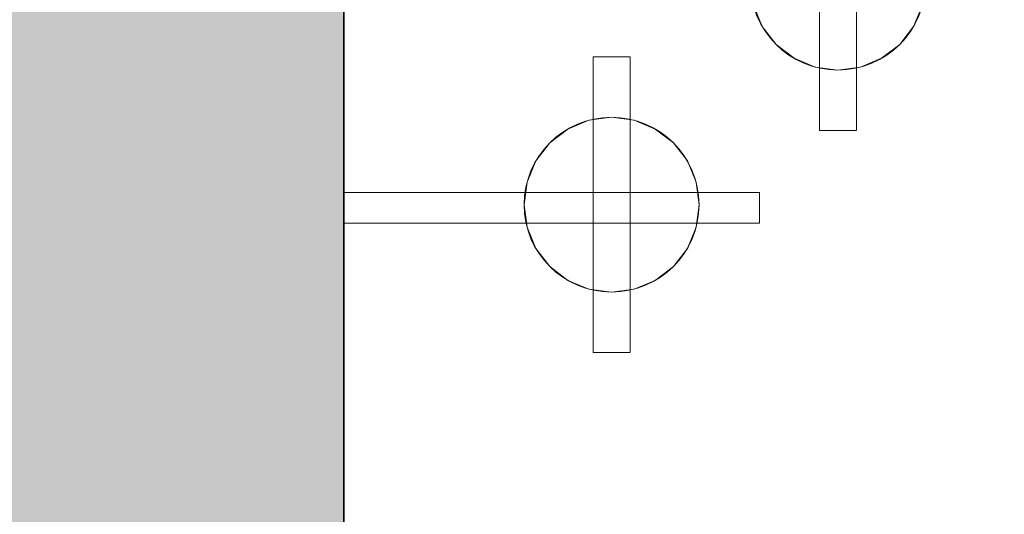
# Model space of a CAD drawing. Units: inches. Extents: x 2696 to 3240, y 1564 to 2310.
# Tile 6 of 76: x 2893.424 to 2903.397, y 1638.544 to 1643.56. Entities that reach past the tile are written whole.
import ezdxf

# ---------------------------------------------------------------- set-up
doc = ezdxf.new("R2010")
doc.units = ezdxf.units.IN
for name, color, linetype, lineweight in [('A-ANNO-DIMS', 3, 'Continuous', 18), ('A-FLOR-FIXT', 8, 'Continuous', 18), ('A-FURN', 251, 'Continuous', 13), ('A-WALL', 7, 'Continuous', 35), ('A-WALL-PATT', 9, 'Continuous', 13)]:
    doc.layers.add(name, color=color, linetype=linetype, lineweight=lineweight)
doc.layers.add('FURNITURE', color=250, linetype='Continuous')
doc.styles.add('TIMES NEW', font='times.ttf')
doc.dimstyles.new('Siddhuu', dxfattribs={"dimtxt": 6, "dimasz": 2.5, "dimexe": 1.25, "dimexo": 0.625, "dimtad": 1, "dimdec": 1, "dimlunit": 4, "dimtxsty": 'TIMES NEW', "dimcen": 2.5, "dimclrd": 256, "dimclre": 1, "dimclrt": 7, "dimadec": 0, "dimazin": 0, "dimtfac": 1, "dimtdec": 1, "dimtmove": 0, "dimatfit": 3, "dimfxl": 1, "dimtolj": 1, "dimlwd": -1, "dimarcsym": 0})

# ---------------------------------------------------------------- blocks, each defined once
blk = doc.blocks.new('A$C1af1f523')
at = {"layer": 'A-FURN'}
for p, q in [((-5.1906, 1.6871), (-5.1901, -1.3115)), ((-5.1906, 1.6871, 0.5), (-5.1901, -1.3115, 0.5)), ((-4.8156, 1.6871), (-4.8151, -1.3115)), ((-4.8156, 1.6871, 0.5), (-4.8151, -1.3115, 0.5)), ((-5.77, -0.2555), (-5.77, -0.2555, 0.5)), ((-4.2353, -0.2555), (-4.2353, -0.2555, 0.5)), ((-5.6292, -0.439), (-5.6292, -0.439, 0.5)), ((-4.3761, -0.439), (-4.3761, -0.439, 0.5)), ((-5.4457, -0.5798), (-5.4457, -0.5798, 0.5)), ((-4.5596, -0.5798), (-4.5596, -0.5798, 0.5)), ((-2.898, -0.5642), (-2.898, -3.5628)), ((-2.898, -0.5642, 0.5), (-2.898, -3.5628, 0.5)), ((-2.898, -0.5642), (-2.898, -0.5642, 0.5)), ((-2.523, -0.5642), (-2.898, -0.5642)), ((-2.523, -0.5642, 0.5), (-2.898, -0.5642, 0.5)), ((-2.523, -0.5642), (-2.523, -3.5628)), ((-2.523, -0.5642, 0.5), (-2.523, -3.5628, 0.5)), ((-2.523, -0.5642), (-2.523, -0.5642, 0.5)), ((-5.232, -0.6683), (-5.232, -0.6683, 0.5)), ((-4.7733, -0.6683), (-4.7733, -0.6683, 0.5)), ((-5.0026, -0.6985), (-5.0026, -0.6985, 0.5)), ((-2.7105, -1.1778), (-2.7105, -1.1778, 0.5)), ((-2.9398, -1.208), (-2.9398, -1.208, 0.5)), ((-2.4812, -1.208), (-2.4812, -1.208, 0.5)), ((-5.1901, -1.3115), (-5.1901, -1.3115, 0.5)), ((-4.8151, -1.3115), (-5.1878, -1.3115)), ((-4.8151, -1.3115, 0.5), (-5.1878, -1.3115, 0.5)), ((-5.1878, -1.3115), (-5.1878, -1.3115, 0.5)), ((-4.8151, -1.3115), (-4.8151, -1.3115, 0.5)), ((-3.1535, -1.2965), (-3.1535, -1.2965, 0.5)), ((-2.2675, -1.2965), (-2.2675, -1.2965, 0.5)), ((-3.337, -1.4373), (-3.337, -1.4373, 0.5)), ((-2.084, -1.4373), (-2.084, -1.4373, 0.5)), ((-3.4778, -1.6208), (-3.4778, -1.6208, 0.5)), ((-1.9432, -1.6208), (-1.9432, -1.6208, 0.5)), ((-3.5664, -1.8345), (-3.5664, -1.8345, 0.5)), ((-1.8547, -1.8345), (-1.8547, -1.8345, 0.5)), ((0, -1.9388), (-4.2094, -1.9388)), ((0, -1.9388, 0.5), (-4.2094, -1.9388, 0.5)), ((-4.2094, -1.9388), (-4.2094, -1.9388, 0.5)), ((-4.2094, -1.9399), (-4.2094, -2.2513)), ((-4.2094, -1.9399, 0.5), (-4.2094, -2.2513, 0.5)), ((-4.2094, -1.9399), (-4.2094, -1.9399, 0.5)), ((-3.5965, -2.0638), (-3.5965, -2.0638, 0.5)), ((-1.8245, -2.0638), (-1.8245, -2.0638, 0.5)), ((0, -2.2513), (-4.2094, -2.2513)), ((0, -2.2513, 0.5), (-4.2094, -2.2513, 0.5)), ((-4.2094, -2.2513), (-4.2094, -2.2513, 0.5)), ((-4.2094, -2.2513), (-4.2094, -2.2524)), ((-4.2094, -2.2513, 0.5), (-4.2094, -2.2524, 0.5)), ((-4.2094, -2.2524), (-4.2094, -2.2524, 0.5)), ((-3.5664, -2.2931), (-3.5664, -2.2931, 0.5)), ((-1.8547, -2.2931), (-1.8547, -2.2931, 0.5)), ((-3.4778, -2.5068), (-3.4778, -2.5068, 0.5)), ((-1.9432, -2.5068), (-1.9432, -2.5068, 0.5)), ((-3.337, -2.6903), (-3.337, -2.6903, 0.5)), ((-2.084, -2.6903), (-2.084, -2.6903, 0.5)), ((-3.1535, -2.8311), (-3.1535, -2.8311, 0.5)), ((-2.2675, -2.8311), (-2.2675, -2.8311, 0.5)), ((-2.9398, -2.9196), (-2.9398, -2.9196, 0.5)), ((-2.7105, -2.9498), (-2.7105, -2.9498, 0.5)), ((-2.4812, -2.9196), (-2.4812, -2.9196, 0.5)), ((-2.898, -3.5628), (-2.898, -3.5628, 0.5)), ((-2.523, -3.5628), (-2.8956, -3.5628)), ((-2.523, -3.5628, 0.5), (-2.8956, -3.5628, 0.5)), ((-2.8956, -3.5628), (-2.8956, -3.5628, 0.5)), ((-2.523, -3.5628), (-2.523, -3.5628, 0.5))]:
    blk.add_line(p, q, dxfattribs=at)
for centre in [(-5.0026, 0.1875), (-5.0026, 0.1875, 0.5), (-2.7105, -2.0638), (-2.7105, -2.0638, 0.5)]:
    blk.add_circle(centre, 0.886, dxfattribs=at)
at = {"layer": 'FURNITURE'}
for p, q in [((0, -1.9388), (0, -1.9388, 0.5)), ((0, -2.2513), (0, -2.2513, 0.5))]:
    blk.add_line(p, q, dxfattribs=at)
at = {"layer": 'A-FURN'}
mesh = blk.add_polyface(dxfattribs=at)
corners = [(-5.1901, -1.3115, 0.5), (-5.1906, 1.6871), (-5.1901, -1.3115), (-5.1906, 1.6871, 0.5)]
mesh.append_faces([[corners[k] for k in face] for face in [(2, 1, 0), (3, 0, 1)]], dxfattribs={"vtx1": -1})
mesh = blk.add_polyface(dxfattribs=at)
corners = [(-4.8151, -1.3115, 0.5), (-4.8156, 1.6871), (-4.8151, -1.3115), (-4.8156, 1.6871, 0.5)]
mesh.append_faces([[corners[k] for k in face] for face in [(2, 1, 0), (3, 0, 1)]], dxfattribs={"vtx1": -1})
mesh = blk.add_polyface(dxfattribs=at)
corners = [(-5.8585, -0.0418, 0.5), (-5.77, -0.2555), (-5.8585, -0.0418), (-5.77, -0.2555, 0.5)]
mesh.append_faces([[corners[k] for k in face] for face in [(2, 1, 0), (3, 0, 1)]], dxfattribs={"vtx1": -1})
mesh = blk.add_polyface(dxfattribs=at)
corners = [(-4.2353, -0.2555, 0.5), (-4.1468, -0.0418), (-4.2353, -0.2555), (-4.1468, -0.0418, 0.5)]
mesh.append_faces([[corners[k] for k in face] for face in [(2, 1, 0), (3, 0, 1)]], dxfattribs={"vtx1": -1})
mesh = blk.add_polyface(dxfattribs=at)
corners = [(-5.77, -0.2555, 0.5), (-5.6292, -0.439), (-5.77, -0.2555), (-5.6292, -0.439, 0.5)]
mesh.append_faces([[corners[k] for k in face] for face in [(2, 1, 0), (3, 0, 1)]], dxfattribs={"vtx1": -1})
mesh = blk.add_polyface(dxfattribs=at)
corners = [(-4.3761, -0.439, 0.5), (-4.2353, -0.2555), (-4.3761, -0.439), (-4.2353, -0.2555, 0.5)]
mesh.append_faces([[corners[k] for k in face] for face in [(2, 1, 0), (3, 0, 1)]], dxfattribs={"vtx1": -1})
mesh = blk.add_polyface(dxfattribs=at)
corners = [(-5.4457, -0.5798, 0.5), (-5.6292, -0.439), (-5.6292, -0.439, 0.5), (-5.4457, -0.5798)]
mesh.append_faces([[corners[k] for k in face] for face in [(2, 1, 0), (3, 0, 1)]], dxfattribs={"vtx1": -1})
mesh = blk.add_polyface(dxfattribs=at)
corners = [(-4.3761, -0.439, 0.5), (-4.5596, -0.5798), (-4.5596, -0.5798, 0.5), (-4.3761, -0.439)]
mesh.append_faces([[corners[k] for k in face] for face in [(2, 1, 0), (3, 0, 1)]], dxfattribs={"vtx1": -1})
mesh = blk.add_polyface(dxfattribs=at)
corners = [(-5.232, -0.6683, 0.5), (-5.4457, -0.5798), (-5.4457, -0.5798, 0.5), (-5.232, -0.6683)]
mesh.append_faces([[corners[k] for k in face] for face in [(2, 1, 0), (3, 0, 1)]], dxfattribs={"vtx1": -1})
mesh = blk.add_polyface(dxfattribs=at)
corners = [(-4.5596, -0.5798, 0.5), (-4.7733, -0.6683), (-4.7733, -0.6683, 0.5), (-4.5596, -0.5798)]
mesh.append_faces([[corners[k] for k in face] for face in [(2, 1, 0), (3, 0, 1)]], dxfattribs={"vtx1": -1})
mesh = blk.add_polyface(dxfattribs=at)
corners = [(-2.898, -3.5628, 0.5), (-2.898, -0.5642), (-2.898, -3.5628), (-2.898, -0.5642, 0.5)]
mesh.append_faces([[corners[k] for k in face] for face in [(2, 1, 0), (3, 0, 1)]], dxfattribs={"vtx1": -1})
mesh = blk.add_polyface(dxfattribs=at)
corners = [(-2.523, -0.5642, 0.5), (-2.898, -0.5642), (-2.898, -0.5642, 0.5), (-2.523, -0.5642)]
mesh.append_faces([[corners[k] for k in face] for face in [(2, 1, 0), (3, 0, 1)]], dxfattribs={"vtx1": -1})
mesh = blk.add_polyface(dxfattribs=at)
corners = [(-2.523, -3.5628, 0.5), (-2.523, -0.5642), (-2.523, -3.5628), (-2.523, -0.5642, 0.5)]
mesh.append_faces([[corners[k] for k in face] for face in [(2, 1, 0), (3, 0, 1)]], dxfattribs={"vtx1": -1})
mesh = blk.add_polyface(dxfattribs=at)
corners = [(-5.0026, -0.6985, 0.5), (-5.232, -0.6683), (-5.232, -0.6683, 0.5), (-5.0026, -0.6985)]
mesh.append_faces([[corners[k] for k in face] for face in [(2, 1, 0), (3, 0, 1)]], dxfattribs={"vtx1": -1})
mesh = blk.add_polyface(dxfattribs=at)
corners = [(-4.7733, -0.6683, 0.5), (-5.0026, -0.6985), (-5.0026, -0.6985, 0.5), (-4.7733, -0.6683)]
mesh.append_faces([[corners[k] for k in face] for face in [(2, 1, 0), (3, 0, 1)]], dxfattribs={"vtx1": -1})
mesh = blk.add_polyface(dxfattribs=at)
corners = [(-2.7105, -1.1778), (-2.9398, -1.208, 0.5), (-2.9398, -1.208), (-2.7105, -1.1778, 0.5)]
mesh.append_faces([[corners[k] for k in face] for face in [(2, 1, 0), (3, 0, 1)]], dxfattribs={"vtx1": -1})
mesh = blk.add_polyface(dxfattribs=at)
corners = [(-2.4812, -1.208), (-2.7105, -1.1778, 0.5), (-2.7105, -1.1778), (-2.4812, -1.208, 0.5)]
mesh.append_faces([[corners[k] for k in face] for face in [(2, 1, 0), (3, 0, 1)]], dxfattribs={"vtx1": -1})
mesh = blk.add_polyface(dxfattribs=at)
corners = [(-2.9398, -1.208), (-3.1535, -1.2965, 0.5), (-3.1535, -1.2965), (-2.9398, -1.208, 0.5)]
mesh.append_faces([[corners[k] for k in face] for face in [(2, 1, 0), (3, 0, 1)]], dxfattribs={"vtx1": -1})
mesh = blk.add_polyface(dxfattribs=at)
corners = [(-2.2675, -1.2965), (-2.4812, -1.208, 0.5), (-2.4812, -1.208), (-2.2675, -1.2965, 0.5)]
mesh.append_faces([[corners[k] for k in face] for face in [(2, 1, 0), (3, 0, 1)]], dxfattribs={"vtx1": -1})
mesh = blk.add_polyface(dxfattribs=at)
corners = [(-4.8151, -1.3115, 0.5), (-5.1878, -1.3115), (-5.1878, -1.3115, 0.5), (-4.8151, -1.3115)]
mesh.append_faces([[corners[k] for k in face] for face in [(2, 1, 0), (3, 0, 1)]], dxfattribs={"vtx1": -1})
mesh = blk.add_polyface(dxfattribs=at)
corners = [(-3.1535, -1.2965), (-3.337, -1.4373, 0.5), (-3.337, -1.4373), (-3.1535, -1.2965, 0.5)]
mesh.append_faces([[corners[k] for k in face] for face in [(2, 1, 0), (3, 0, 1)]], dxfattribs={"vtx1": -1})
mesh = blk.add_polyface(dxfattribs=at)
corners = [(-2.084, -1.4373), (-2.2675, -1.2965, 0.5), (-2.2675, -1.2965), (-2.084, -1.4373, 0.5)]
mesh.append_faces([[corners[k] for k in face] for face in [(2, 1, 0), (3, 0, 1)]], dxfattribs={"vtx1": -1})
mesh = blk.add_polyface(dxfattribs=at)
corners = [(-3.337, -1.4373, 0.5), (-3.4778, -1.6208), (-3.337, -1.4373), (-3.4778, -1.6208, 0.5)]
mesh.append_faces([[corners[k] for k in face] for face in [(2, 1, 0), (3, 0, 1)]], dxfattribs={"vtx1": -1})
mesh = blk.add_polyface(dxfattribs=at)
corners = [(-1.9432, -1.6208, 0.5), (-2.084, -1.4373), (-1.9432, -1.6208), (-2.084, -1.4373, 0.5)]
mesh.append_faces([[corners[k] for k in face] for face in [(2, 1, 0), (3, 0, 1)]], dxfattribs={"vtx1": -1})
mesh = blk.add_polyface(dxfattribs=at)
corners = [(-3.4778, -1.6208, 0.5), (-3.5664, -1.8345), (-3.4778, -1.6208), (-3.5664, -1.8345, 0.5)]
mesh.append_faces([[corners[k] for k in face] for face in [(2, 1, 0), (3, 0, 1)]], dxfattribs={"vtx1": -1})
mesh = blk.add_polyface(dxfattribs=at)
corners = [(-1.8547, -1.8345, 0.5), (-1.9432, -1.6208), (-1.8547, -1.8345), (-1.9432, -1.6208, 0.5)]
mesh.append_faces([[corners[k] for k in face] for face in [(2, 1, 0), (3, 0, 1)]], dxfattribs={"vtx1": -1})
mesh = blk.add_polyface(dxfattribs=at)
corners = [(-3.5664, -1.8345, 0.5), (-3.5965, -2.0638), (-3.5664, -1.8345), (-3.5965, -2.0638, 0.5)]
mesh.append_faces([[corners[k] for k in face] for face in [(2, 1, 0), (3, 0, 1)]], dxfattribs={"vtx1": -1})
mesh = blk.add_polyface(dxfattribs=at)
corners = [(-1.8245, -2.0638, 0.5), (-1.8547, -1.8345), (-1.8245, -2.0638), (-1.8547, -1.8345, 0.5)]
mesh.append_faces([[corners[k] for k in face] for face in [(2, 1, 0), (3, 0, 1)]], dxfattribs={"vtx1": -1})
mesh = blk.add_polyface(dxfattribs=at)
corners = [(0, -1.9388, 0.5), (-4.2094, -1.9388), (-4.2094, -1.9388, 0.5), (0, -1.9388)]
mesh.append_faces([[corners[k] for k in face] for face in [(2, 1, 0), (3, 0, 1)]], dxfattribs={"vtx1": -1})
mesh = blk.add_polyface(dxfattribs=at)
corners = [(-4.2094, -2.2524, 0.5), (-4.2094, -2.2513), (-4.2094, -2.2524), (-4.2094, -1.9399), (-4.2094, -1.9399, 0.5), (-4.2094, -2.2513, 0.5)]
mesh.append_faces([[corners[k] for k in face] for face in [(3, 0, 1), (4, 0, 3)]], dxfattribs={"vtx0": -1, "vtx1": -1})
mesh.append_faces([[corners[k] for k in face] for face in [(2, 1, 0), (5, 0, 4)]], dxfattribs={"vtx1": -1})
mesh = blk.add_polyface(dxfattribs=at)
corners = [(-3.5965, -2.0638, 0.5), (-3.5664, -2.2931), (-3.5965, -2.0638), (-3.5664, -2.2931, 0.5)]
mesh.append_faces([[corners[k] for k in face] for face in [(2, 1, 0), (3, 0, 1)]], dxfattribs={"vtx1": -1})
mesh = blk.add_polyface(dxfattribs=at)
corners = [(-1.8547, -2.2931, 0.5), (-1.8245, -2.0638), (-1.8547, -2.2931), (-1.8245, -2.0638, 0.5)]
mesh.append_faces([[corners[k] for k in face] for face in [(2, 1, 0), (3, 0, 1)]], dxfattribs={"vtx1": -1})
mesh = blk.add_polyface(dxfattribs=at)
corners = [(0, -2.2513, 0.5), (-4.2094, -2.2513), (-4.2094, -2.2513, 0.5), (0, -2.2513)]
mesh.append_faces([[corners[k] for k in face] for face in [(2, 1, 0), (3, 0, 1)]], dxfattribs={"vtx1": -1})
mesh = blk.add_polyface(dxfattribs=at)
corners = [(-3.5664, -2.2931, 0.5), (-3.4778, -2.5068), (-3.5664, -2.2931), (-3.4778, -2.5068, 0.5)]
mesh.append_faces([[corners[k] for k in face] for face in [(2, 1, 0), (3, 0, 1)]], dxfattribs={"vtx1": -1})
mesh = blk.add_polyface(dxfattribs=at)
corners = [(-1.9432, -2.5068, 0.5), (-1.8547, -2.2931), (-1.9432, -2.5068), (-1.8547, -2.2931, 0.5)]
mesh.append_faces([[corners[k] for k in face] for face in [(2, 1, 0), (3, 0, 1)]], dxfattribs={"vtx1": -1})
mesh = blk.add_polyface(dxfattribs=at)
corners = [(-3.4778, -2.5068, 0.5), (-3.337, -2.6903), (-3.4778, -2.5068), (-3.337, -2.6903, 0.5)]
mesh.append_faces([[corners[k] for k in face] for face in [(2, 1, 0), (3, 0, 1)]], dxfattribs={"vtx1": -1})
mesh = blk.add_polyface(dxfattribs=at)
corners = [(-2.084, -2.6903, 0.5), (-1.9432, -2.5068), (-2.084, -2.6903), (-1.9432, -2.5068, 0.5)]
mesh.append_faces([[corners[k] for k in face] for face in [(2, 1, 0), (3, 0, 1)]], dxfattribs={"vtx1": -1})
mesh = blk.add_polyface(dxfattribs=at)
corners = [(-3.1535, -2.8311, 0.5), (-3.337, -2.6903), (-3.337, -2.6903, 0.5), (-3.1535, -2.8311)]
mesh.append_faces([[corners[k] for k in face] for face in [(2, 1, 0), (3, 0, 1)]], dxfattribs={"vtx1": -1})
mesh = blk.add_polyface(dxfattribs=at)
corners = [(-2.084, -2.6903, 0.5), (-2.2675, -2.8311), (-2.2675, -2.8311, 0.5), (-2.084, -2.6903)]
mesh.append_faces([[corners[k] for k in face] for face in [(2, 1, 0), (3, 0, 1)]], dxfattribs={"vtx1": -1})
mesh = blk.add_polyface(dxfattribs=at)
corners = [(-2.9398, -2.9196, 0.5), (-3.1535, -2.8311), (-3.1535, -2.8311, 0.5), (-2.9398, -2.9196)]
mesh.append_faces([[corners[k] for k in face] for face in [(2, 1, 0), (3, 0, 1)]], dxfattribs={"vtx1": -1})
mesh = blk.add_polyface(dxfattribs=at)
corners = [(-2.2675, -2.8311, 0.5), (-2.4812, -2.9196), (-2.4812, -2.9196, 0.5), (-2.2675, -2.8311)]
mesh.append_faces([[corners[k] for k in face] for face in [(2, 1, 0), (3, 0, 1)]], dxfattribs={"vtx1": -1})
mesh = blk.add_polyface(dxfattribs=at)
corners = [(-2.7105, -2.9498, 0.5), (-2.9398, -2.9196), (-2.9398, -2.9196, 0.5), (-2.7105, -2.9498)]
mesh.append_faces([[corners[k] for k in face] for face in [(2, 1, 0), (3, 0, 1)]], dxfattribs={"vtx1": -1})
mesh = blk.add_polyface(dxfattribs=at)
corners = [(-2.4812, -2.9196, 0.5), (-2.7105, -2.9498), (-2.7105, -2.9498, 0.5), (-2.4812, -2.9196)]
mesh.append_faces([[corners[k] for k in face] for face in [(2, 1, 0), (3, 0, 1)]], dxfattribs={"vtx1": -1})
mesh = blk.add_polyface(dxfattribs=at)
corners = [(-2.523, -3.5628, 0.5), (-2.8956, -3.5628), (-2.8956, -3.5628, 0.5), (-2.523, -3.5628)]
mesh.append_faces([[corners[k] for k in face] for face in [(2, 1, 0), (3, 0, 1)]], dxfattribs={"vtx1": -1})
blk = doc.blocks.new('*D36')
at = {"layer": 'A-ANNO-DIMS', "color": 1, "lineweight": -2, "transparency": 16777216}
for p, q in [((3008.2374, 1629.3861), (3008.2374, 1619.4611)), ((3070.2374, 1629.3861), (3070.2374, 1619.4611))]:
    blk.add_line(p, q, dxfattribs=at)
at = {"layer": 'A-ANNO-DIMS', "transparency": 16777216}
for p, q in [((3008.2374, 1620.7111), (2894.7181, 1620.7111)), ((3067.7374, 1620.7111), (3010.7374, 1620.7111))]:
    blk.add_line(p, q, dxfattribs=at)
for points in [[(3010.7374, 1621.1278), (3010.7374, 1620.2944), (3008.2374, 1620.7111)], [(3067.7374, 1621.1278), (3067.7374, 1620.2944), (3070.2374, 1620.7111)]]:
    blk.add_solid(points, dxfattribs=at)
at = {"layer": 'Defpoints', "color": 0, "transparency": 16777216}
for p in [(3008.2374, 1630.0111), (3070.2374, 1630.0111), (3008.2374, 1620.7111)]:
    blk.add_point(p, dxfattribs=at)
at = {"layer": 'A-ANNO-DIMS', "color": 7, "transparency": 16777216, "insert": (2950.2277, 1624.4031), "char_height": 6, "attachment_point": 5, "style": 'TIMES NEW'}
blk.add_mtext('\\A1;BALCONY DOOR 5\'-2" TYP.', dxfattribs=at)
blk = doc.blocks.new('*D57')
at = {"layer": 'A-ANNO-DIMS', "color": 1, "lineweight": -2, "transparency": 16777216}
for p, q in [((2754.6114, 2018.5761), (2754.6114, 1568.9511)), ((2956.7088, 2018.5761), (2956.7088, 1568.9511))]:
    blk.add_line(p, q, dxfattribs=at)
at = {"layer": 'A-ANNO-DIMS', "transparency": 16777216}
blk.add_line((2757.1114, 1570.2011), (2954.2088, 1570.2011), dxfattribs=at)
for points in [[(2757.1114, 1570.6178), (2757.1114, 1569.7844), (2754.6114, 1570.2011)], [(2954.2088, 1570.6178), (2954.2088, 1569.7844), (2956.7088, 1570.2011)]]:
    blk.add_solid(points, dxfattribs=at)
at = {"layer": 'Defpoints', "color": 0, "transparency": 16777216}
for p in [(2754.6114, 2019.2011), (2956.7088, 2019.2011), (2956.7088, 1570.2011)]:
    blk.add_point(p, dxfattribs=at)
at = {"layer": 'A-ANNO-DIMS', "color": 7, "transparency": 16777216, "insert": (2855.6601, 1573.878), "char_height": 6, "attachment_point": 5, "style": 'TIMES NEW'}
blk.add_mtext('\\A1;16\'-10"', dxfattribs=at)
blk = doc.blocks.new('*D69')
at = {"layer": 'A-ANNO-DIMS', "color": 1, "lineweight": -2, "transparency": 16777216}
for p, q in [((2841.889, 2261.5761), (2841.889, 1568.9511)), ((2905.9101, 2261.5761), (2905.9101, 1568.9511))]:
    blk.add_line(p, q, dxfattribs=at)
at = {"layer": 'A-ANNO-DIMS', "transparency": 16777216}
blk.add_line((2844.389, 1570.2011), (2903.4101, 1570.2011), dxfattribs=at)
for points in [[(2844.389, 1570.6178), (2844.389, 1569.7844), (2841.889, 1570.2011)], [(2903.4101, 1570.6178), (2903.4101, 1569.7844), (2905.9101, 1570.2011)]]:
    blk.add_solid(points, dxfattribs=at)
at = {"layer": 'Defpoints', "color": 0, "transparency": 16777216}
for p in [(2841.889, 2262.2011), (2905.9101, 2262.2011), (2905.9101, 1570.2011)]:
    blk.add_point(p, dxfattribs=at)
at = {"layer": 'A-ANNO-DIMS', "color": 7, "transparency": 16777216, "insert": (2873.8995, 1573.878), "char_height": 6, "attachment_point": 5, "style": 'TIMES NEW'}
blk.add_mtext('\\A1;5\'-4"', dxfattribs=at)

msp = doc.modelspace()

# ---------------------------------------------------------------- hatches: boundary and pattern name
at = {"layer": 'A-WALL-PATT', "transparency": 33554556}
h = msp.add_hatch(color=256, dxfattribs=at)
h.dxf.hatch_style = 1
h.paths.add_polyline_path([(2879.1114, 2253.2011), (2905.9101, 2253.2011), (2905.9101, 2262.2011), (2841.889, 2262.2011), (2841.889, 2253.2011), (2870.1114, 2253.2011), (2870.1114, 2176.6011), (2965.7088, 2176.6011), (2965.7088, 2206.7011), (2973.5828, 2206.7011), (2973.5828, 2215.7011), (2965.7088, 2215.7011), (2965.7088, 2262.2011), (2929.9101, 2262.2011), (2929.9101, 2253.2011), (2956.7088, 2253.2011), (2956.7088, 2185.6011), (2879.1114, 2185.6011)])
h.paths.add_polyline_path([(2782.8338, 2262.2011), (2745.6114, 2262.2011), (2745.6114, 2228.7287), (2754.6114, 2228.7287), (2754.6114, 2253.2011), (2782.8338, 2253.2011)])
h.paths.add_polyline_path([(2754.6114, 2136.2011), (2965.7088, 2136.2011), (2965.7088, 2145.2011), (2879.1114, 2145.2011), (2879.1114, 2147.0735), (2877.3397, 2147.0735), (2870.1114, 2147.0735), (2870.1114, 2145.2011), (2754.6114, 2145.2011), (2754.6114, 2169.6735), (2745.6114, 2169.6735), (2745.6114, 2000.2011), (2754.6114, 2000.2011), (2754.6114, 2019.2011), (2849.0828, 2019.2011), (2849.0828, 2023.7011), (2841.2088, 2023.7011), (2841.2088, 2051.8271), (2836.7088, 2051.8271), (2836.7088, 2023.7011), (2754.6114, 2023.7011), (2754.6114, 2091.2011), (2836.7088, 2091.2011), (2836.7088, 2087.8271), (2841.2088, 2087.8271), (2841.2088, 2095.7011), (2754.6114, 2095.7011)])
h.paths.add_polyline_path([(2965.7088, 2136.2011), (2956.7088, 2136.2011), (2956.7088, 2023.7011), (2885.0828, 2023.7011), (2885.0828, 2019.2011), (2956.7088, 2019.2011), (2956.7088, 1950.5751), (2965.7088, 1950.5751), (2965.7088, 1980.2011), (2973.5828, 1980.2011), (2973.5828, 1989.2011), (2965.7088, 1989.2011)])
h.paths.add_polyline_path([(2754.6114, 1906.7011), (2880.2088, 1906.7011), (2884.7088, 1906.7011), (2956.7088, 1906.7011), (2956.7088, 1792.7011), (2944.7088, 1792.7011), (2944.7088, 1783.7011), (2956.7088, 1783.7011), (2956.7088, 1740.2011), (2884.7088, 1740.2011), (2884.7088, 1783.7011), (2896.7088, 1783.7011), (2896.7088, 1792.7011), (2884.7088, 1792.7011), (2884.7088, 1846.7011), (2880.2088, 1846.7011), (2880.2088, 1740.2011), (2754.6114, 1740.2011), (2754.6114, 1777.2011), (2745.6114, 1777.2011), (2745.6114, 1692.7011), (2754.6114, 1692.7011), (2754.6114, 1731.2011), (2956.7088, 1731.2011), (2956.7088, 1723.3271), (2965.7088, 1723.3271), (2965.7088, 1884.2011), (2973.5828, 1884.2011), (2973.5828, 1893.2011), (2965.7088, 1893.2011), (2965.7088, 1914.5751), (2956.7088, 1914.5751), (2956.7088, 1911.2011), (2754.6114, 1911.2011), (2754.6114, 1930.2011), (2745.6114, 1930.2011), (2745.6114, 1817.2011), (2754.6114, 1817.2011), (2754.6114, 1854.2011), (2826.6114, 1854.2011), (2826.6114, 1868.8271), (2822.1114, 1868.8271), (2822.1114, 1858.7011), (2754.6114, 1858.7011)])
h.paths.add_polyline_path([(2965.7088, 1656.2011), (3008.2374, 1656.2011), (3008.2374, 1665.2011), (2965.7088, 1665.2011), (2965.7088, 1693.3271), (2956.7088, 1693.3271), (2956.7088, 1686.2011), (2934.5828, 1686.2011), (2934.5828, 1681.7011), (2956.7088, 1681.7011), (2956.7088, 1614.2011), (2896.7088, 1614.2011), (2896.7088, 1681.7011), (2904.5828, 1681.7011), (2904.5828, 1686.2011), (2892.2088, 1686.2011), (2892.2088, 1614.2011), (2858.4101, 1614.2011), (2858.4101, 1605.2011), (2965.7088, 1605.2011)])
h.paths.add_polyline_path([(2788.4101, 1614.2011), (2754.6114, 1614.2011), (2754.6114, 1652.7011), (2745.6114, 1652.7011), (2745.6114, 1605.2011), (2788.4101, 1605.2011)])
h.paths.add_polyline_path([(3199.6114, 1633.0476), (3190.6114, 1633.0476), (3190.6114, 1614.2011), (3082.6114, 1614.2011), (3082.6114, 1665.2011), (3070.2374, 1665.2011), (3070.2374, 1656.2011), (3078.1114, 1656.2011), (3078.1114, 1605.2011), (3199.6114, 1605.2011)])
h.paths.add_polyline_path([(3199.6114, 1702.0476), (3190.6114, 1702.0476), (3190.6114, 1699.7011), (3106.6114, 1699.7011), (3106.6114, 1747.7011), (3190.6114, 1747.7011), (3190.6114, 1752.2011), (3082.6114, 1752.2011), (3082.6114, 1760.0751), (3078.1114, 1760.0751), (3078.1114, 1747.7011), (3102.1114, 1747.7011), (3102.1114, 1699.7011), (3078.1114, 1699.7011), (3078.1114, 1695.2011), (3190.6114, 1695.2011), (3190.6114, 1676.3546), (3199.6114, 1676.3546)])
h.paths.add_polyline_path([(3199.6114, 1783.2011), (3190.6114, 1783.2011), (3190.6114, 1745.3546), (3199.6114, 1745.3546)])
h.paths.add_polyline_path([(3082.6114, 1884.2011), (3190.6114, 1884.2011), (3190.6114, 1853.2011), (3199.6114, 1853.2011), (3199.6114, 1901.7011), (3190.6114, 1901.7011), (3190.6114, 1893.2011), (3005.5828, 1893.2011), (3005.5828, 1891.2811), (3005.5828, 1884.2011), (3078.1114, 1884.2011), (3078.1114, 1792.0751), (3082.6114, 1792.0751)])
h.paths.add_polyline_path([(3199.6114, 1994.7011), (3190.6114, 1994.7011), (3190.6114, 1989.2011), (3073.7088, 1989.2011), (3073.7088, 2034.2011), (3069.2088, 2034.2011), (3069.2088, 1989.2011), (3005.5828, 1989.2011), (3005.5828, 1980.2011), (3190.6114, 1980.2011), (3190.6114, 1971.7011), (3199.6114, 1971.7011)])
h.paths.add_polyline_path([(3199.6114, 2155.2011), (3190.6114, 2155.2011), (3190.6114, 2064.7011), (3199.6114, 2064.7011)])
h.paths.add_polyline_path([(3190.6114, 2074.7011), (3106.6114, 2074.7011), (3106.6114, 2122.7011), (3190.6114, 2122.7011), (3190.6114, 2127.2011), (3082.7088, 2127.2011), (3082.7088, 2135.0751), (3073.7088, 2135.0751), (3073.7088, 2122.7011), (3102.1114, 2122.7011), (3102.1114, 2074.7011), (3069.2088, 2074.7011), (3069.2088, 2070.2011), (3190.6114, 2070.2011)])
h.paths.add_polyline_path([(3082.7088, 2253.2011), (3190.6114, 2253.2011), (3190.6114, 2225.2011), (3199.6114, 2225.2011), (3199.6114, 2262.2011), (3073.7088, 2262.2011), (3073.7088, 2215.7011), (3035.5828, 2215.7011), (3035.5828, 2206.7011), (3073.7088, 2206.7011), (3073.7088, 2171.0751), (3082.7088, 2171.0751)])

# ---------------------------------------------------------------- linework, layer by layer
at = {"layer": 'A-WALL'}
msp.add_line((2896.7088, 1681.7011), (2896.7088, 1614.2011), dxfattribs=at)

# ---------------------------------------------------------------- block references
at = {"layer": 'A-FLOR-FIXT', "xscale": -1}
msp.add_blockref('A$C1af1f523', (2896.7088, 1643.7478), dxfattribs=at)

# ---------------------------------------------------------------- dimensions: what is measured, and where the dimension line sits
at = {"layer": 'A-ANNO-DIMS'}
for base, p1, p2, picture, middle in [((2905.9101, 1570.2011), (2841.889, 2262.2011), (2905.9101, 2262.2011), '*D69', (2873.8995, 1573.878)), ((2956.7088, 1570.2011), (2754.6114, 2019.2011), (2956.7088, 2019.2011), '*D57', (2855.6601, 1573.878))]:
    dim = msp.add_linear_dim(base=base, p1=p1, p2=p2, dimstyle='Siddhuu', override={"dimdec": 1, "dimlfac": 1, "dimrnd": 0, "dimzin": 1, "dimdsep": 46, "dimlunit": 4, "dimfrac": 2}, dxfattribs=at)
    dim.commit()
    dim.dimension.update_dxf_attribs({"geometry": picture, "text_midpoint": middle})
dim = msp.add_linear_dim(base=(3008.2374, 1620.7111), p1=(3070.2374, 1630.0111), p2=(3008.2374, 1630.0111), angle=180, text='BALCONY DOOR <> TYP.', dimstyle='Siddhuu', override={"dimdec": 1, "dimlfac": 1, "dimrnd": 0, "dimzin": 1, "dimdsep": 46, "dimlunit": 4, "dimfrac": 2}, dxfattribs=at)
dim.commit()
dim.dimension.update_dxf_attribs({"geometry": '*D36', "text_midpoint": (2950.2277, 1624.4031)})

doc.saveas('drawing.dxf')
